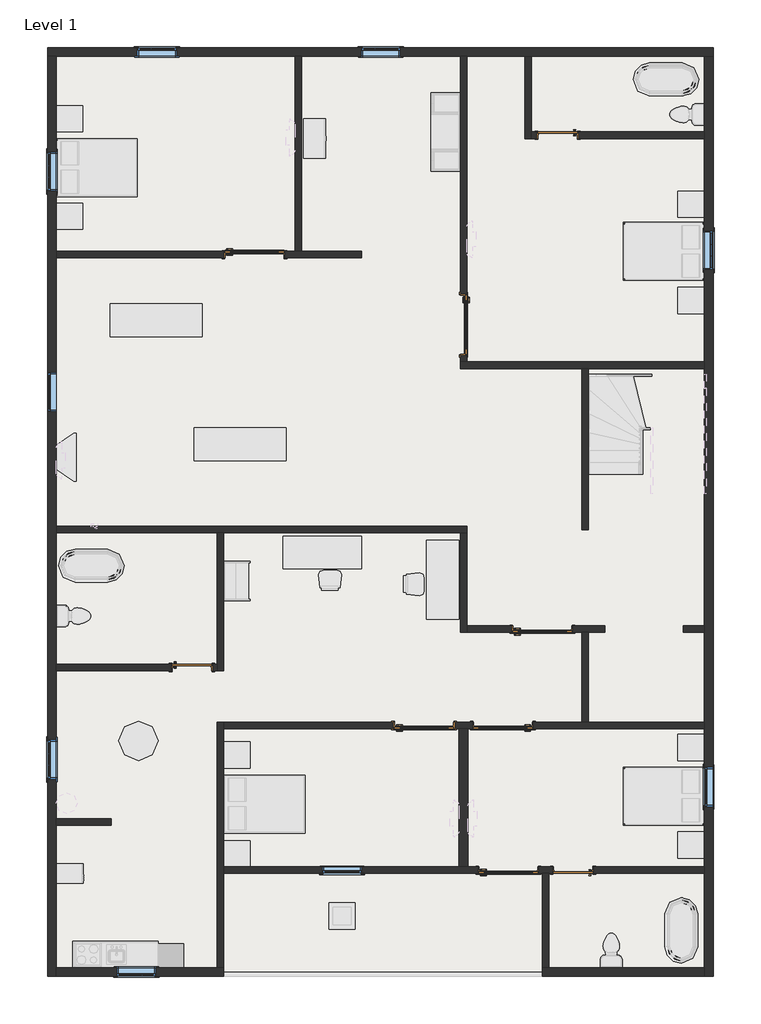
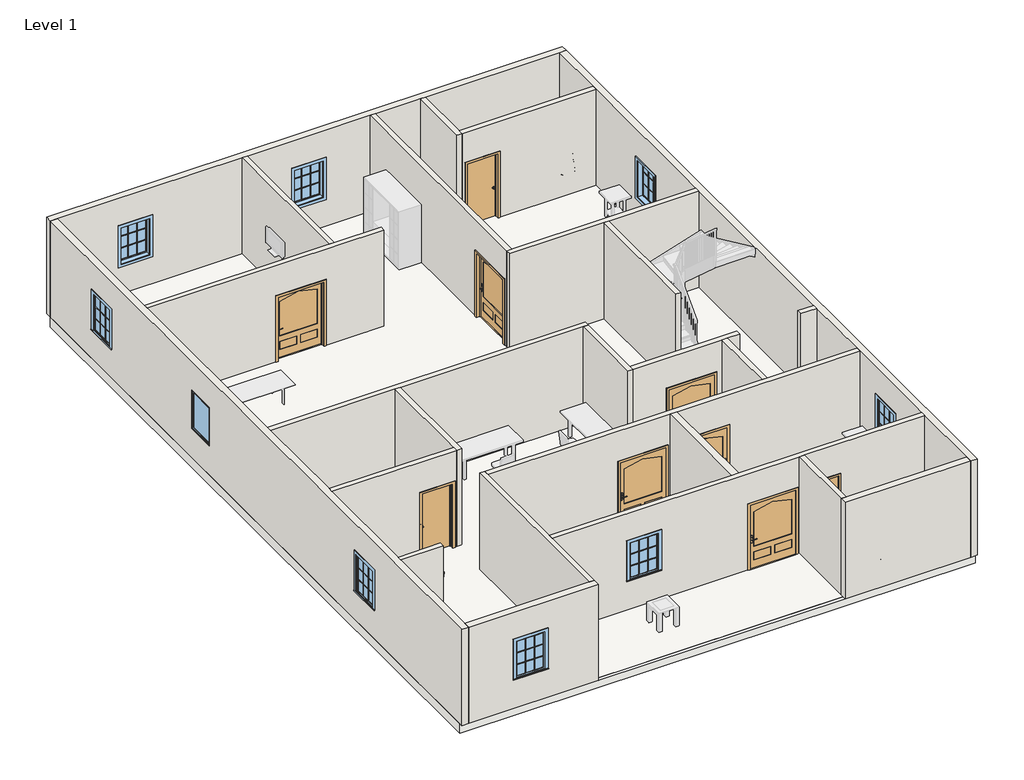
# One storey, part 1 of 2: 25 walls, 9 doors, 9 windows, 1 slab.
"""IFC4 building model written with IfcOpenShell, lengths in millimetres."""

from ifc_helpers import new_model, si_unit, frame, origin, origin_with_axes, place, context, project, spatial, polyline, outline, extrude, faceted_brep, transform, mapped, element, save
from components import door_483975e0, door_8e627b7d, door_2171c7d8, door_acdcadbb, window_29c06734, window_5c190c7e, window_e2841890

model = new_model("IFC4")

# Units and contexts
model_context = context("Model", 3, world=origin())
ifc_project = project(units=[si_unit("LENGTHUNIT", "METRE", prefix="MILLI")], contexts=[model_context])

# Site, building, storey
site = spatial("IfcSite", under=ifc_project)
building = spatial("IfcBuilding", under=site)
storey = spatial("IfcBuildingStorey", under=building, Name="Level 1", Elevation=0.0)

# Doors
placement = place(None, origin())
door_shape = door_483975e0(model_context)
element("IfcDoor", 1, ObjectType="54\" x 80\"", at=placement, inside=storey, context=model_context, shape_type="MappedRepresentation", body=[
    mapped(door_shape, transform((-4346.7860513, -470.0045948, 0.0), x_axis=(1.0, 0.0, 0.0), y_axis=(0.0, 1.0, 0.0), z_axis=(0.0, 0.0, 1.0))),
])
element("IfcDoor", 2, ObjectType="54\" x 80\"", at=placement, inside=storey, context=model_context, shape_type="MappedRepresentation", body=[
    mapped(door_shape, transform((-10112.5860513, 10458.3454052, 0.0), x_axis=(-1.0, 0.0, 0.0), y_axis=(0.0, -1.0, 0.0), z_axis=(0.0, 0.0, 1.0))),
])
element("IfcDoor", 3, ObjectType="54\" x 80\"", at=placement, inside=storey, context=model_context, shape_type="MappedRepresentation", body=[
    mapped(door_shape, transform((-5258.0110513, 8829.5704052, 0.0), x_axis=(0.0, 1.0, 0.0), y_axis=(-1.0, 0.0, 0.0), z_axis=(0.0, 0.0, 1.0))),
])
door_2_shape = door_8e627b7d(model_context)
element("IfcDoor", 4, ObjectType="54\" x 80\"", at=placement, inside=storey, context=model_context, shape_type="MappedRepresentation", body=[
    mapped(door_2_shape, transform((-4219.7860513, -3822.8045948, 0.0), x_axis=(-1.0, 0.0, 0.0), y_axis=(0.0, -1.0, 0.0), z_axis=(0.0, 0.0, 1.0))),
])
element("IfcDoor", 5, ObjectType="54\" x 80\"", at=placement, inside=storey, context=model_context, shape_type="MappedRepresentation", body=[
    mapped(door_2_shape, transform((-6175.5860513, -470.0045948, 0.0), x_axis=(-1.0, 0.0, 0.0), y_axis=(0.0, -1.0, 0.0), z_axis=(0.0, 0.0, 1.0))),
])
element("IfcDoor", 6, ObjectType="54\" x 80\"", at=placement, inside=storey, context=model_context, shape_type="MappedRepresentation", body=[
    mapped(door_2_shape, transform((-3432.3860513, 1765.1954052, 0.0), x_axis=(-1.0, 0.0, 0.0), y_axis=(0.0, -1.0, 0.0), z_axis=(0.0, 0.0, 1.0))),
])
door_3_shape = door_2171c7d8(model_context)
element("IfcDoor", 7, ObjectType="Door-Interior-Single-Flush_Panel-Wood : 36\" x 80\"", at=placement, inside=storey, context=model_context, shape_type="MappedRepresentation", body=[
    mapped(door_3_shape, transform((-2721.1860513, -3822.8045948, 0.0), x_axis=(-1.0, 0.0, 0.0), y_axis=(0.0, -1.0, 0.0), z_axis=(0.0, 0.0, 1.0))),
])
element("IfcDoor", 8, ObjectType="Door-Interior-Single-Flush_Panel-Wood : 36\" x 80\"", at=placement, inside=storey, context=model_context, shape_type="MappedRepresentation", body=[
    mapped(door_3_shape, transform((-11560.3860513, 882.5454052, 0.0), x_axis=(1.0, 0.0, 0.0), y_axis=(0.0, 1.0, 0.0), z_axis=(0.0, 0.0, 1.0))),
])
door_4_shape = door_acdcadbb(model_context)
element("IfcDoor", 9, ObjectType="Door-Interior-Single-Flush_Panel-Wood : 36\" x 80\"", at=placement, inside=storey, context=model_context, shape_type="MappedRepresentation", body=[
    mapped(door_4_shape, transform((-3076.7860513, 13226.9454052, 0.0), x_axis=(-1.0, 0.0, 0.0), y_axis=(0.0, -1.0, 0.0), z_axis=(0.0, 0.0, 1.0))),
])

# Slab
element("IfcSlab", 10, ObjectType="Generic - 12\"", at=placement, inside=storey, context=model_context, shape_type="SweptSolid", body=[
    extrude(outline(polyline([(530.0139487, 15052.5704052), (530.0139487, -6181.8295948), (-14913.1860513, -6181.8295948), (-14913.1860513, 15052.5704052), (530.0139487, 15052.5704052)])), frame((0.0, 0.0, -304.8), z_axis=(0.0, 0.0, 1.0), x_axis=(1.0, 0.0, 0.0)), (0.0, 0.0, 1.0), 304.8),
])

# Walls
element("IfcWall", 11, ObjectType="Generic - 8\"", at=placement, inside=storey, context=model_context, shape_type="Brep", body=[
    faceted_brep([(-14913.1860513, 15052.5704052, 0.0), (-14709.9860513, 15052.5704052, 0.0), (-9172.7860513, 15052.5704052, 0.0), (-9020.3860513, 15052.5704052, 0.0), (-5337.3860513, 15052.5704052, 0.0), (-5184.9860513, 15052.5704052, 0.0), (-3838.7860513, 15052.5704052, 0.0), (-3686.3860513, 15052.5704052, 0.0), (326.8139487, 15052.5704052, 0.0), (530.0139487, 15052.5704052, 0.0), (530.0139487, 15052.5704052, 3048.0), (326.8139487, 15052.5704052, 3048.0), (-3686.3860513, 15052.5704052, 3048.0), (-3838.7860513, 15052.5704052, 3048.0), (-5184.9860513, 15052.5704052, 3048.0), (-5337.3860513, 15052.5704052, 3048.0), (-9020.3860513, 15052.5704052, 3048.0), (-9172.7860513, 15052.5704052, 3048.0), (-14709.9860513, 15052.5704052, 3048.0), (-14913.1860513, 15052.5704052, 3048.0), (-11915.9860513, 15052.5704052, 2133.6), (-11915.9860513, 15052.5704052, 914.4), (-12830.3860513, 15052.5704052, 914.4), (-12830.3860513, 15052.5704052, 2133.6), (-6721.6860513, 15052.5704052, 2133.6), (-6721.6860513, 15052.5704052, 914.4), (-7636.0860513, 15052.5704052, 914.4), (-7636.0860513, 15052.5704052, 2133.6), (-14913.1860513, 15255.7704052, 0.0), (-14913.1860513, 15255.7704052, 3048.0), (530.0139487, 15255.7704052, 3048.0), (530.0139487, 15255.7704052, 0.0), (-11915.9860513, 15255.7704052, 2133.6), (-12830.3860513, 15255.7704052, 2133.6), (-12830.3860513, 15255.7704052, 914.4), (-11915.9860513, 15255.7704052, 914.4), (-6721.6860513, 15255.7704052, 2133.6), (-7636.0860513, 15255.7704052, 2133.6), (-7636.0860513, 15255.7704052, 914.4), (-6721.6860513, 15255.7704052, 914.4)], [[[0, 1, 2, 3, 4, 5, 6, 7, 8, 9, 10, 11, 12, 13, 14, 15, 16, 17, 18, 19], [20, 21, 22, 23], [24, 25, 26, 27]], [[28, 29, 30, 31], [32, 33, 34, 35], [36, 37, 38, 39]], [[9, 8, 7, 6, 5, 4, 3, 2, 1, 0, 28, 31]], [[19, 18, 17, 16, 15, 14, 13, 12, 11, 10, 30, 29]], [[10, 9, 31, 30]], [[0, 19, 29, 28]], [[21, 20, 32, 35]], [[22, 21, 35, 34]], [[23, 22, 34, 33]], [[20, 23, 33, 32]], [[25, 24, 36, 39]], [[26, 25, 39, 38]], [[27, 26, 38, 37]], [[24, 27, 37, 36]]]),
])
element("IfcWall", 12, ObjectType="Generic - 8\"", at=placement, inside=storey, context=model_context, shape_type="Brep", body=[
    faceted_brep([(326.8139487, 15052.5704052, 0.0), (326.8139487, 13299.9704052, 0.0), (326.8139487, 13147.5704052, 0.0), (326.8139487, 7965.9704052, 0.0), (326.8139487, 7813.5704052, 0.0), (326.8139487, 1844.5704052, 0.0), (326.8139487, 1692.1704052, 0.0), (326.8139487, -390.6295948, 0.0), (326.8139487, -543.0295948, 0.0), (326.8139487, -3743.4295948, 0.0), (326.8139487, -3895.8295948, 0.0), (326.8139487, -6080.2295948, 0.0), (326.8139487, -6283.4295948, 0.0), (326.8139487, -6283.4295948, 3048.0), (326.8139487, -6080.2295948, 3048.0), (326.8139487, -3895.8295948, 3048.0), (326.8139487, -3743.4295948, 3048.0), (326.8139487, -543.0295948, 3048.0), (326.8139487, -390.6295948, 3048.0), (326.8139487, 1692.1704052, 3048.0), (326.8139487, 1844.5704052, 3048.0), (326.8139487, 7813.5704052, 3048.0), (326.8139487, 7965.9704052, 3048.0), (326.8139487, 13147.5704052, 3048.0), (326.8139487, 13299.9704052, 3048.0), (326.8139487, 15052.5704052, 3048.0), (326.8139487, -1432.0295948, 2133.6), (326.8139487, -2346.4295948, 2133.6), (326.8139487, -2346.4295948, 914.4), (326.8139487, -1432.0295948, 914.4), (326.8139487, 10099.5704052, 2133.6), (326.8139487, 10099.5704052, 914.4), (326.8139487, 11013.9704052, 914.4), (326.8139487, 11013.9704052, 2133.6), (530.0139487, 15052.5704052, 0.0), (530.0139487, 15052.5704052, 3048.0), (530.0139487, -6283.4295948, 3048.0), (530.0139487, -6283.4295948, 0.0), (530.0139487, -1432.0295948, 2133.6), (530.0139487, -1432.0295948, 914.4), (530.0139487, -2346.4295948, 914.4), (530.0139487, -2346.4295948, 2133.6), (530.0139487, 10099.5704052, 2133.6), (530.0139487, 11013.9704052, 2133.6), (530.0139487, 11013.9704052, 914.4), (530.0139487, 10099.5704052, 914.4)], [[[0, 1, 2, 3, 4, 5, 6, 7, 8, 9, 10, 11, 12, 13, 14, 15, 16, 17, 18, 19, 20, 21, 22, 23, 24, 25], [26, 27, 28, 29], [30, 31, 32, 33]], [[34, 35, 36, 37], [38, 39, 40, 41], [42, 43, 44, 45]], [[12, 11, 10, 9, 8, 7, 6, 5, 4, 3, 2, 1, 0, 34, 37]], [[25, 24, 23, 22, 21, 20, 19, 18, 17, 16, 15, 14, 13, 36, 35]], [[0, 25, 35, 34]], [[13, 12, 37, 36]], [[39, 38, 26, 29]], [[40, 39, 29, 28]], [[41, 40, 28, 27]], [[38, 41, 27, 26]], [[31, 30, 42, 45]], [[32, 31, 45, 44]], [[33, 32, 44, 43]], [[30, 33, 43, 42]]]),
])
element("IfcWall", 13, ObjectType="Generic - 8\"", at=placement, inside=storey, context=model_context, shape_type="Brep", body=[
    faceted_brep([(-14913.1860513, 15052.5704052, 0.0), (-14913.1860513, -6283.4295948, 0.0), (-14913.1860513, -6283.4295948, 3048.0), (-14913.1860513, 15052.5704052, 3048.0), (-14913.1860513, 12842.7704052, 2133.6), (-14913.1860513, 11928.3704052, 2133.6), (-14913.1860513, 11928.3704052, 914.4), (-14913.1860513, 12842.7704052, 914.4), (-14913.1860513, -797.0295948, 2133.6), (-14913.1860513, -1711.4295948, 2133.6), (-14913.1860513, -1711.4295948, 914.4), (-14913.1860513, -797.0295948, 914.4), (-14913.1860513, 7724.6704052, 2133.6), (-14913.1860513, 6810.2704052, 2133.6), (-14913.1860513, 6810.2704052, 914.4), (-14913.1860513, 7724.6704052, 914.4), (-14709.9860513, 15052.5704052, 0.0), (-14709.9860513, 15052.5704052, 3048.0), (-14709.9860513, 10531.3704052, 3048.0), (-14709.9860513, 10378.9704052, 3048.0), (-14709.9860513, 4155.9704052, 3048.0), (-14709.9860513, 4003.5704052, 3048.0), (-14709.9860513, 955.5704052, 3048.0), (-14709.9860513, 803.1704052, 3048.0), (-14709.9860513, -2625.8295948, 3048.0), (-14709.9860513, -2778.2295948, 3048.0), (-14709.9860513, -6080.2295948, 3048.0), (-14709.9860513, -6283.4295948, 3048.0), (-14709.9860513, -6283.4295948, 0.0), (-14709.9860513, -6080.2295948, 0.0), (-14709.9860513, -2778.2295948, 0.0), (-14709.9860513, -2625.8295948, 0.0), (-14709.9860513, 803.1704052, 0.0), (-14709.9860513, 955.5704052, 0.0), (-14709.9860513, 4003.5704052, 0.0), (-14709.9860513, 4155.9704052, 0.0), (-14709.9860513, 10378.9704052, 0.0), (-14709.9860513, 10531.3704052, 0.0), (-14709.9860513, 12842.7704052, 2133.6), (-14709.9860513, 12842.7704052, 914.4), (-14709.9860513, 11928.3704052, 914.4), (-14709.9860513, 11928.3704052, 2133.6), (-14709.9860513, -797.0295948, 2133.6), (-14709.9860513, -797.0295948, 914.4), (-14709.9860513, -1711.4295948, 914.4), (-14709.9860513, -1711.4295948, 2133.6), (-14709.9860513, 7724.6704052, 2133.6), (-14709.9860513, 7724.6704052, 914.4), (-14709.9860513, 6810.2704052, 914.4), (-14709.9860513, 6810.2704052, 2133.6)], [[[0, 1, 2, 3], [4, 5, 6, 7], [8, 9, 10, 11], [12, 13, 14, 15]], [[16, 17, 18, 19, 20, 21, 22, 23, 24, 25, 26, 27, 28, 29, 30, 31, 32, 33, 34, 35, 36, 37], [38, 39, 40, 41], [42, 43, 44, 45], [46, 47, 48, 49]], [[1, 0, 16, 37, 36, 35, 34, 33, 32, 31, 30, 29, 28]], [[3, 2, 27, 26, 25, 24, 23, 22, 21, 20, 19, 18, 17]], [[0, 3, 17, 16]], [[2, 1, 28, 27]], [[39, 38, 4, 7]], [[40, 39, 7, 6]], [[41, 40, 6, 5]], [[38, 41, 5, 4]], [[43, 42, 8, 11]], [[44, 43, 11, 10]], [[45, 44, 10, 9]], [[42, 45, 9, 8]], [[47, 46, 12, 15]], [[48, 47, 15, 14]], [[49, 48, 14, 13]], [[46, 49, 13, 12]]]),
])
element("IfcWall", 14, ObjectType="Generic - 8\"", at=placement, inside=storey, context=model_context, shape_type="Brep", body=[
    faceted_brep([(-14709.9860513, -6283.4295948, 0.0), (-10823.7860513, -6283.4295948, 0.0), (-10823.7860513, -6283.4295948, 3048.0), (-14709.9860513, -6283.4295948, 3048.0), (-13312.9860513, -6283.4295948, 2133.6), (-12398.5860513, -6283.4295948, 2133.6), (-12398.5860513, -6283.4295948, 914.4), (-13312.9860513, -6283.4295948, 914.4), (-14709.9860513, -6080.2295948, 0.0), (-14709.9860513, -6080.2295948, 3048.0), (-10976.1860513, -6080.2295948, 3048.0), (-10823.7860513, -6080.2295948, 3048.0), (-10823.7860513, -6080.2295948, 0.0), (-10976.1860513, -6080.2295948, 0.0), (-13312.9860513, -6080.2295948, 2133.6), (-13312.9860513, -6080.2295948, 914.4), (-12398.5860513, -6080.2295948, 914.4), (-12398.5860513, -6080.2295948, 2133.6)], [[[0, 1, 2, 3], [4, 5, 6, 7]], [[8, 9, 10, 11, 12, 13], [14, 15, 16, 17]], [[1, 0, 8, 13, 12]], [[3, 2, 11, 10, 9]], [[0, 3, 9, 8]], [[2, 1, 12, 11]], [[15, 14, 4, 7]], [[16, 15, 7, 6]], [[17, 16, 6, 5]], [[14, 17, 5, 4]]]),
])
element("IfcWall", 15, ObjectType="Generic - 8\"", at=placement, inside=storey, context=model_context, shape_type="SweptSolid", body=[
    extrude(outline(polyline([(-5362.7860513, -3743.4295948), (-5362.7860513, -543.0295948), (-5159.5860513, -543.0295948), (-5159.5860513, -3743.4295948), (-5362.7860513, -3743.4295948)])), origin_with_axes(), (0.0, 0.0, 1.0), 3048.0),
])
element("IfcWall", 16, ObjectType="Generic - 8\"", at=placement, inside=storey, context=model_context, shape_type="Brep", body=[
    faceted_brep([(-3432.3860513, -6283.4295948, 0.0), (326.8139487, -6283.4295948, 0.0), (326.8139487, -6283.4295948, 3048.0), (-3432.3860513, -6283.4295948, 3048.0), (-3432.3860513, -6080.2295948, 0.0), (-3432.3860513, -6080.2295948, 3048.0), (-3279.9860513, -6080.2295948, 3048.0), (326.8139487, -6080.2295948, 3048.0), (326.8139487, -6080.2295948, 0.0), (-3279.9860513, -6080.2295948, 0.0)], [[[0, 1, 2, 3]], [[4, 5, 6, 7, 8, 9]], [[1, 0, 4, 9, 8]], [[3, 2, 7, 6, 5]], [[2, 1, 8, 7]], [[0, 3, 5, 4]]]),
])
element("IfcWall", 17, ObjectType="INNER WALL", at=placement, inside=storey, context=model_context, shape_type="SweptSolid", body=[
    extrude(outline(polyline([(-9172.7860513, 10531.3704052), (-9172.7860513, 15052.5704052), (-9020.3860513, 15052.5704052), (-9020.3860513, 10531.3704052), (-9172.7860513, 10531.3704052)])), origin_with_axes(), (0.0, 0.0, 1.0), 3048.0),
])
element("IfcWall", 18, ObjectType="INNER WALL", at=placement, inside=storey, context=model_context, shape_type="Brep", body=[
    faceted_brep([(-14709.9860513, 10531.3704052, 3048.0), (-9172.7860513, 10531.3704052, 3048.0), (-9020.3860513, 10531.3704052, 3048.0), (-7623.3860513, 10531.3704052, 3048.0), (-7623.3860513, 10531.3704052, 0.0), (-9020.3860513, 10531.3704052, 0.0), (-9172.7860513, 10531.3704052, 0.0), (-9401.3860513, 10531.3704052, 0.0), (-9401.3860513, 10531.3704052, 2057.4), (-10823.7860513, 10531.3704052, 2057.4), (-10823.7860513, 10531.3704052, 0.0), (-14709.9860513, 10531.3704052, 0.0), (-7623.3860513, 10378.9704052, 3048.0), (-14709.9860513, 10378.9704052, 3048.0), (-14709.9860513, 10378.9704052, 0.0), (-10823.7860513, 10378.9704052, 0.0), (-10823.7860513, 10378.9704052, 2057.4), (-9401.3860513, 10378.9704052, 2057.4), (-9401.3860513, 10378.9704052, 0.0), (-7623.3860513, 10378.9704052, 0.0)], [[[0, 1, 2, 3, 4, 5, 6, 7, 8, 9, 10, 11]], [[12, 13, 14, 15, 16, 17, 18, 19]], [[4, 19, 18, 7, 6, 5]], [[14, 11, 10, 15]], [[3, 2, 1, 0, 13, 12]], [[4, 3, 12, 19]], [[0, 11, 14, 13]], [[9, 16, 15, 10]], [[16, 9, 8, 17]], [[17, 8, 7, 18]]]),
])
element("IfcWall", 19, ObjectType="INNER WALL", at=placement, inside=storey, context=model_context, shape_type="SweptSolid", body=[
    extrude(outline(polyline([(7965.9704052, 3048.0), (15052.5704052, 3048.0), (15052.5704052, 0.0), (9540.7704052, 0.0), (9540.7704052, 2057.4), (8118.3704052, 2057.4), (8118.3704052, 0.0), (7965.9704052, 0.0), (7965.9704052, 3048.0)])), frame((-5337.3860513, 0.0, 0.0), z_axis=(1.0, 0.0, 0.0), x_axis=(0.0, 1.0, 0.0)), (0.0, 0.0, 1.0), 152.4),
])
element("IfcWall", 20, ObjectType="INNER WALL", at=placement, inside=storey, context=model_context, shape_type="Brep", body=[
    faceted_brep([(-5337.3860513, 7813.5704052, 0.0), (-2517.9860513, 7813.5704052, 0.0), (-2365.5860513, 7813.5704052, 0.0), (326.8139487, 7813.5704052, 0.0), (326.8139487, 7813.5704052, 3048.0), (-2365.5860513, 7813.5704052, 3048.0), (-2517.9860513, 7813.5704052, 3048.0), (-5337.3860513, 7813.5704052, 3048.0), (-5337.3860513, 7965.9704052, 0.0), (-5337.3860513, 7965.9704052, 3048.0), (-5184.9860513, 7965.9704052, 3048.0), (326.8139487, 7965.9704052, 3048.0), (326.8139487, 7965.9704052, 0.0), (-5184.9860513, 7965.9704052, 0.0)], [[[0, 1, 2, 3, 4, 5, 6, 7]], [[8, 9, 10, 11, 12, 13]], [[3, 2, 1, 0, 8, 13, 12]], [[7, 6, 5, 4, 11, 10, 9]], [[4, 3, 12, 11]], [[0, 7, 9, 8]]]),
])
element("IfcWall", 21, ObjectType="INNER WALL", at=placement, inside=storey, context=model_context, shape_type="SweptSolid", body=[
    extrude(outline(polyline([(-2517.9860513, 4079.7704052), (-2517.9860513, 7813.5704052), (-2365.5860513, 7813.5704052), (-2365.5860513, 4079.7704052), (-2517.9860513, 4079.7704052)])), origin_with_axes(), (0.0, 0.0, 1.0), 3048.0),
])
element("IfcWall", 22, ObjectType="INNER WALL", at=placement, inside=storey, context=model_context, shape_type="Brep", body=[
    faceted_brep([(-14709.9860513, 4003.5704052, 0.0), (-10976.1860513, 4003.5704052, 0.0), (-10823.7860513, 4003.5704052, 0.0), (-5337.3860513, 4003.5704052, 0.0), (-5184.9860513, 4003.5704052, 0.0), (-5184.9860513, 4003.5704052, 3048.0), (-5337.3860513, 4003.5704052, 3048.0), (-10823.7860513, 4003.5704052, 3048.0), (-10976.1860513, 4003.5704052, 3048.0), (-14709.9860513, 4003.5704052, 3048.0), (-14709.9860513, 4155.9704052, 0.0), (-14709.9860513, 4155.9704052, 3048.0), (-5184.9860513, 4155.9704052, 3048.0), (-5184.9860513, 4155.9704052, 0.0)], [[[0, 1, 2, 3, 4, 5, 6, 7, 8, 9]], [[10, 11, 12, 13]], [[4, 3, 2, 1, 0, 10, 13]], [[9, 8, 7, 6, 5, 12, 11]], [[0, 9, 11, 10]], [[5, 4, 13, 12]]]),
])
element("IfcWall", 23, ObjectType="INNER WALL", at=placement, inside=storey, context=model_context, shape_type="Brep", body=[
    faceted_brep([(-5337.3860513, 4003.5704052, 0.0), (-5337.3860513, 1692.1704052, 0.0), (-5337.3860513, 1692.1704052, 3048.0), (-5337.3860513, 4003.5704052, 3048.0), (-5184.9860513, 4003.5704052, 0.0), (-5184.9860513, 4003.5704052, 3048.0), (-5184.9860513, 1844.5704052, 3048.0), (-5184.9860513, 1692.1704052, 3048.0), (-5184.9860513, 1692.1704052, 0.0), (-5184.9860513, 1844.5704052, 0.0)], [[[0, 1, 2, 3]], [[4, 5, 6, 7, 8, 9]], [[1, 0, 4, 9, 8]], [[3, 2, 7, 6, 5]], [[0, 3, 5, 4]], [[2, 1, 8, 7]]]),
])
element("IfcWall", 24, ObjectType="INNER WALL", at=placement, inside=storey, context=model_context, shape_type="Brep", body=[
    faceted_brep([(-1984.5860513, 1692.1704052, 0.0), (-1984.5860513, 1692.1704052, 3048.0), (-2365.5860513, 1692.1704052, 3048.0), (-2517.9860513, 1692.1704052, 3048.0), (-5184.9860513, 1692.1704052, 3048.0), (-5184.9860513, 1692.1704052, 0.0), (-4143.5860513, 1692.1704052, 0.0), (-4143.5860513, 1692.1704052, 2057.4), (-2721.1860513, 1692.1704052, 2057.4), (-2721.1860513, 1692.1704052, 0.0), (-2517.9860513, 1692.1704052, 0.0), (-2365.5860513, 1692.1704052, 0.0), (-1984.5860513, 1844.5704052, 3048.0), (-1984.5860513, 1844.5704052, 0.0), (-2721.1860513, 1844.5704052, 0.0), (-2721.1860513, 1844.5704052, 2057.4), (-4143.5860513, 1844.5704052, 2057.4), (-4143.5860513, 1844.5704052, 0.0), (-5184.9860513, 1844.5704052, 0.0), (-5184.9860513, 1844.5704052, 3048.0)], [[[0, 1, 2, 3, 4, 5, 6, 7, 8, 9, 10, 11]], [[12, 13, 14, 15, 16, 17, 18, 19]], [[13, 0, 11, 10, 9, 14]], [[5, 18, 17, 6]], [[1, 0, 13, 12]], [[4, 3, 2, 1, 12, 19]], [[5, 4, 19, 18]], [[16, 7, 6, 17]], [[7, 16, 15, 8]], [[8, 15, 14, 9]]]),
])
element("IfcWall", 25, ObjectType="INNER WALL", at=placement, inside=storey, context=model_context, shape_type="SweptSolid", body=[
    extrude(outline(polyline([(-2517.9860513, -390.6295948), (-2517.9860513, 1692.1704052), (-2365.5860513, 1692.1704052), (-2365.5860513, -390.6295948), (-2517.9860513, -390.6295948)])), origin_with_axes(), (0.0, 0.0, 1.0), 3048.0),
])
element("IfcWall", 26, ObjectType="INNER WALL", at=placement, inside=storey, context=model_context, shape_type="SweptSolid", body=[
    extrude(outline(polyline([(-3279.9860513, -3895.8295948), (-3279.9860513, -6080.2295948), (-3432.3860513, -6080.2295948), (-3432.3860513, -3895.8295948), (-3279.9860513, -3895.8295948)])), origin_with_axes(), (0.0, 0.0, 1.0), 3048.0),
])
element("IfcWall", 27, ObjectType="INNER WALL", at=placement, inside=storey, context=model_context, shape_type="Brep", body=[
    faceted_brep([(-10823.7860513, -6080.2295948, 0.0), (-10823.7860513, -3895.8295948, 0.0), (-10823.7860513, -3743.4295948, 0.0), (-10823.7860513, -543.0295948, 0.0), (-10823.7860513, -390.6295948, 0.0), (-10823.7860513, -390.6295948, 3048.0), (-10823.7860513, -543.0295948, 3048.0), (-10823.7860513, -3743.4295948, 3048.0), (-10823.7860513, -3895.8295948, 3048.0), (-10823.7860513, -6080.2295948, 3048.0), (-10976.1860513, -6080.2295948, 0.0), (-10976.1860513, -6080.2295948, 3048.0), (-10976.1860513, -390.6295948, 3048.0), (-10976.1860513, -390.6295948, 0.0)], [[[0, 1, 2, 3, 4, 5, 6, 7, 8, 9]], [[10, 11, 12, 13]], [[4, 3, 2, 1, 0, 10, 13]], [[9, 8, 7, 6, 5, 12, 11]], [[5, 4, 13, 12]], [[0, 9, 11, 10]]]),
])
element("IfcWall", 28, ObjectType="INNER WALL", at=placement, inside=storey, context=model_context, shape_type="Brep", body=[
    faceted_brep([(326.8139487, -543.0295948, 3048.0), (-5159.5860513, -543.0295948, 3048.0), (-5362.7860513, -543.0295948, 3048.0), (-10823.7860513, -543.0295948, 3048.0), (-10823.7860513, -543.0295948, 0.0), (-6886.7860513, -543.0295948, 0.0), (-6886.7860513, -543.0295948, 2057.4), (-5464.3860513, -543.0295948, 2057.4), (-5464.3860513, -543.0295948, 0.0), (-5362.7860513, -543.0295948, 0.0), (-5159.5860513, -543.0295948, 0.0), (-5057.9860513, -543.0295948, 0.0), (-5057.9860513, -543.0295948, 2057.4), (-3635.5860513, -543.0295948, 2057.4), (-3635.5860513, -543.0295948, 0.0), (326.8139487, -543.0295948, 0.0), (-10823.7860513, -390.6295948, 3048.0), (-2517.9860513, -390.6295948, 3048.0), (-2365.5860513, -390.6295948, 3048.0), (326.8139487, -390.6295948, 3048.0), (326.8139487, -390.6295948, 0.0), (-2365.5860513, -390.6295948, 0.0), (-2517.9860513, -390.6295948, 0.0), (-3635.5860513, -390.6295948, 0.0), (-3635.5860513, -390.6295948, 2057.4), (-5057.9860513, -390.6295948, 2057.4), (-5057.9860513, -390.6295948, 0.0), (-5464.3860513, -390.6295948, 0.0), (-5464.3860513, -390.6295948, 2057.4), (-6886.7860513, -390.6295948, 2057.4), (-6886.7860513, -390.6295948, 0.0), (-10823.7860513, -390.6295948, 0.0)], [[[0, 1, 2, 3, 4, 5, 6, 7, 8, 9, 10, 11, 12, 13, 14, 15]], [[16, 17, 18, 19, 20, 21, 22, 23, 24, 25, 26, 27, 28, 29, 30, 31]], [[4, 31, 30, 5]], [[20, 15, 14, 23, 22, 21]], [[26, 11, 10, 9, 8, 27]], [[3, 2, 1, 0, 19, 18, 17, 16]], [[4, 3, 16, 31]], [[0, 15, 20, 19]], [[13, 24, 23, 14]], [[24, 13, 12, 25]], [[25, 12, 11, 26]], [[29, 6, 5, 30]], [[6, 29, 28, 7]], [[7, 28, 27, 8]]]),
])
element("IfcWall", 29, ObjectType="INNER WALL", at=placement, inside=storey, context=model_context, shape_type="Brep", body=[
    faceted_brep([(-10823.7860513, -3743.4295948, 3048.0), (-5362.7860513, -3743.4295948, 3048.0), (-5159.5860513, -3743.4295948, 3048.0), (326.8139487, -3743.4295948, 3048.0), (326.8139487, -3743.4295948, 0.0), (-2238.5860513, -3743.4295948, 0.0), (-2238.5860513, -3743.4295948, 2057.4), (-3203.7860513, -3743.4295948, 2057.4), (-3203.7860513, -3743.4295948, 0.0), (-3508.5860513, -3743.4295948, 0.0), (-3508.5860513, -3743.4295948, 2057.4), (-4930.9860513, -3743.4295948, 2057.4), (-4930.9860513, -3743.4295948, 0.0), (-5159.5860513, -3743.4295948, 0.0), (-5362.7860513, -3743.4295948, 0.0), (-10823.7860513, -3743.4295948, 0.0), (-8537.7860513, -3743.4295948, 2133.6), (-8537.7860513, -3743.4295948, 914.4), (-7623.3860513, -3743.4295948, 914.4), (-7623.3860513, -3743.4295948, 2133.6), (326.8139487, -3895.8295948, 3048.0), (-3279.9860513, -3895.8295948, 3048.0), (-3432.3860513, -3895.8295948, 3048.0), (-10823.7860513, -3895.8295948, 3048.0), (-10823.7860513, -3895.8295948, 0.0), (-4930.9860513, -3895.8295948, 0.0), (-4930.9860513, -3895.8295948, 2057.4), (-3508.5860513, -3895.8295948, 2057.4), (-3508.5860513, -3895.8295948, 0.0), (-3432.3860513, -3895.8295948, 0.0), (-3279.9860513, -3895.8295948, 0.0), (-3203.7860513, -3895.8295948, 0.0), (-3203.7860513, -3895.8295948, 2057.4), (-2238.5860513, -3895.8295948, 2057.4), (-2238.5860513, -3895.8295948, 0.0), (326.8139487, -3895.8295948, 0.0), (-8537.7860513, -3895.8295948, 2133.6), (-7623.3860513, -3895.8295948, 2133.6), (-7623.3860513, -3895.8295948, 914.4), (-8537.7860513, -3895.8295948, 914.4)], [[[0, 1, 2, 3, 4, 5, 6, 7, 8, 9, 10, 11, 12, 13, 14, 15], [16, 17, 18, 19]], [[20, 21, 22, 23, 24, 25, 26, 27, 28, 29, 30, 31, 32, 33, 34, 35], [36, 37, 38, 39]], [[24, 15, 14, 13, 12, 25]], [[4, 35, 34, 5]], [[28, 9, 8, 31, 30, 29]], [[3, 2, 1, 0, 23, 22, 21, 20]], [[0, 15, 24, 23]], [[4, 3, 20, 35]], [[11, 26, 25, 12]], [[26, 11, 10, 27]], [[27, 10, 9, 28]], [[7, 32, 31, 8]], [[32, 7, 6, 33]], [[33, 6, 5, 34]], [[17, 16, 36, 39]], [[18, 17, 39, 38]], [[19, 18, 38, 37]], [[16, 19, 37, 36]]]),
])
element("IfcWall", 30, ObjectType="INNER WALL", at=placement, inside=storey, context=model_context, shape_type="Brep", body=[
    faceted_brep([(-10976.1860513, 4003.5704052, 0.0), (-10976.1860513, 955.5704052, 0.0), (-10976.1860513, 803.1704052, 0.0), (-10976.1860513, 803.1704052, 3048.0), (-10976.1860513, 955.5704052, 3048.0), (-10976.1860513, 4003.5704052, 3048.0), (-10823.7860513, 4003.5704052, 0.0), (-10823.7860513, 4003.5704052, 3048.0), (-10823.7860513, 803.1704052, 3048.0), (-10823.7860513, 803.1704052, 0.0)], [[[0, 1, 2, 3, 4, 5]], [[6, 7, 8, 9]], [[2, 1, 0, 6, 9]], [[5, 4, 3, 8, 7]], [[0, 5, 7, 6]], [[3, 2, 9, 8]]]),
])
element("IfcWall", 31, ObjectType="INNER WALL", at=placement, inside=storey, context=model_context, shape_type="SweptSolid", body=[
    extrude(outline(polyline([(3048.0, -10976.1860513), (3048.0, -14709.9860513), (0.0, -14709.9860513), (0.0, -12042.9860513), (2057.4, -12042.9860513), (2057.4, -11077.7860513), (0.0, -11077.7860513), (0.0, -10976.1860513), (3048.0, -10976.1860513)])), frame((0.0, 803.1704052, 0.0), z_axis=(0.0, 1.0, 0.0), x_axis=(0.0, 0.0, 1.0)), (0.0, 0.0, 1.0), 152.4),
])
element("IfcWall", 32, ObjectType="INNER WALL", at=placement, inside=storey, context=model_context, shape_type="SweptSolid", body=[
    extrude(outline(polyline([(326.8139487, 1692.1704052), (-155.7860513, 1692.1704052), (-155.7860513, 1844.5704052), (326.8139487, 1844.5704052), (326.8139487, 1692.1704052)])), origin_with_axes(), (0.0, 0.0, 1.0), 3048.0),
])
element("IfcWall", 33, ObjectType="INNER WALL", at=placement, inside=storey, context=model_context, shape_type="Brep", body=[
    faceted_brep([(-3838.7860513, 15052.5704052, 0.0), (-3838.7860513, 13147.5704052, 0.0), (-3838.7860513, 13147.5704052, 3048.0), (-3838.7860513, 15052.5704052, 3048.0), (-3686.3860513, 15052.5704052, 0.0), (-3686.3860513, 15052.5704052, 3048.0), (-3686.3860513, 13299.9704052, 3048.0), (-3686.3860513, 13147.5704052, 3048.0), (-3686.3860513, 13147.5704052, 0.0), (-3686.3860513, 13299.9704052, 0.0)], [[[0, 1, 2, 3]], [[4, 5, 6, 7, 8, 9]], [[1, 0, 4, 9, 8]], [[3, 2, 7, 6, 5]], [[0, 3, 5, 4]], [[2, 1, 8, 7]]]),
])
element("IfcWall", 34, ObjectType="INNER WALL", at=placement, inside=storey, context=model_context, shape_type="SweptSolid", body=[
    extrude(outline(polyline([(3048.0, 326.8139487), (3048.0, -3686.3860513), (0.0, -3686.3860513), (0.0, -3559.3860513), (2057.4, -3559.3860513), (2057.4, -2594.1860513), (0.0, -2594.1860513), (0.0, 326.8139487), (3048.0, 326.8139487)])), frame((0.0, 13147.5704052, 0.0), z_axis=(0.0, 1.0, 0.0), x_axis=(0.0, 0.0, 1.0)), (0.0, 0.0, 1.0), 152.4),
])
element("IfcWall", 35, ObjectType="INNER WALL", at=placement, inside=storey, context=model_context, shape_type="SweptSolid", body=[
    extrude(outline(polyline([(-14709.9860513, -2625.8295948), (-13439.9860513, -2625.8295948), (-13439.9860513, -2778.2295948), (-14709.9860513, -2778.2295948), (-14709.9860513, -2625.8295948)])), origin_with_axes(), (0.0, 0.0, 1.0), 3048.0),
])

# Windows
window_shape = window_29c06734(model_context)
element("IfcWindow", 36, ObjectType="Casement 3x3 with Trim : 36\" x 48\"", at=placement, inside=storey, context=model_context, shape_type="MappedRepresentation", body=[
    mapped(window_shape, transform((-12855.7860513, -6181.8295948, 0.0), x_axis=(-1.0, 0.0, 0.0), y_axis=(0.0, -1.0, 0.0), z_axis=(0.0, 0.0, 1.0))),
])
element("IfcWindow", 37, ObjectType="Casement 3x3 with Trim : 36\" x 48\"", at=placement, inside=storey, context=model_context, shape_type="MappedRepresentation", body=[
    mapped(window_shape, transform((428.4139487, -1889.2295948, 0.0), x_axis=(0.0, 1.0, 0.0), y_axis=(-1.0, 0.0, 0.0), z_axis=(0.0, 0.0, 1.0))),
])
element("IfcWindow", 38, ObjectType="Casement 3x3 with Trim : 36\" x 48\"", at=placement, inside=storey, context=model_context, shape_type="MappedRepresentation", body=[
    mapped(window_shape, transform((428.4139487, 10556.7704052, 0.0), x_axis=(0.0, -1.0, 0.0), y_axis=(1.0, 0.0, 0.0), z_axis=(0.0, 0.0, 1.0))),
])
element("IfcWindow", 39, ObjectType="Casement 3x3 with Trim : 36\" x 48\"", at=placement, inside=storey, context=model_context, shape_type="MappedRepresentation", body=[
    mapped(window_shape, transform((-12373.1860513, 15154.1704052, 0.0), x_axis=(1.0, 0.0, 0.0), y_axis=(0.0, 1.0, 0.0), z_axis=(0.0, 0.0, 1.0))),
])
element("IfcWindow", 40, ObjectType="Casement 3x3 with Trim : 36\" x 48\"", at=placement, inside=storey, context=model_context, shape_type="MappedRepresentation", body=[
    mapped(window_shape, transform((-14811.5860513, 12385.5704052, 0.0), x_axis=(0.0, 1.0, 0.0), y_axis=(-1.0, 0.0, 0.0), z_axis=(0.0, 0.0, 1.0))),
])
element("IfcWindow", 41, ObjectType="Casement 3x3 with Trim : 36\" x 48\"", at=placement, inside=storey, context=model_context, shape_type="MappedRepresentation", body=[
    mapped(window_shape, transform((-14811.5860513, -1254.2295948, 0.0), x_axis=(0.0, 1.0, 0.0), y_axis=(-1.0, 0.0, 0.0), z_axis=(0.0, 0.0, 1.0))),
])
element("IfcWindow", 42, ObjectType="Casement 3x3 with Trim : 36\" x 48\"", at=placement, inside=storey, context=model_context, shape_type="MappedRepresentation", body=[
    mapped(window_shape, transform((-7178.8860513, 15154.1704052, 0.0), x_axis=(1.0, 0.0, 0.0), y_axis=(0.0, 1.0, 0.0), z_axis=(0.0, 0.0, 1.0))),
])
window_2_shape = window_5c190c7e(model_context)
element("IfcWindow", 43, ObjectType="Casement 3x3 with Trim : 36\" x 48\"", at=placement, inside=storey, context=model_context, shape_type="MappedRepresentation", body=[
    mapped(window_2_shape, transform((-8080.5860513, -3819.6295948, 0.0), x_axis=(-1.0, 0.0, 0.0), y_axis=(0.0, -1.0, 0.0), z_axis=(0.0, 0.0, 1.0))),
])
window_3_shape = window_e2841890(model_context)
element("IfcWindow", 44, ObjectType="Fixed : 36\" x 48\"", at=placement, inside=storey, context=model_context, shape_type="MappedRepresentation", body=[
    mapped(window_3_shape, transform((-14811.5860513, 7305.5704052, 0.0), x_axis=(0.0, 1.0, 0.0), y_axis=(-1.0, 0.0, 0.0), z_axis=(0.0, 0.0, 1.0))),
])

save(model, "model.ifc")

# Revit data of these elements
# Type "54\" x 80\""
#   Type Mark = "8"
#   Assembly Code = "B2030100"
#   Analytic Construction = "French door, wood frame with single glass"
#   Threshold Offset [instance default] = 0' - 0 1/2"
#   Thickness = 0' - 1 3/8"
#   Thermal Resistance (R) = 1.0696 (h·ft²·°F)/BTU
#   Swing Angle [instance default] = 90.00°
#   Stiles = 0' - 4 3/4"
#   Rough Width = 4' - 8"
#   Rough Height = 6' - 9"
#   Radius = 4' - 4.00625"
#   Lock Rail = 0' - 7 1/8"
#   Height = 6' - 8"
#   Width = 4' - 6"
#   Heat Transfer Coefficient (U) = 0.9350 BTU/(h·ft²·°F)
#   Door Offset [instance default] = 0' - 0"
#   Bottom Rail = 0' - 9 1/2"
#   Threshold [instance default] = yes
#   Function = 1
#   Exterior Trim [instance default] = yes
#   Trim Material = Cherry
#   Threshold Material = Cherry
#   Panel Material = Cherry
#   Glazing = Glass
#   Frame Material = Cherry
#   Door Handle Material = Aluminum
#   Visual Light Transmittance = 0
#   Solar Heat Gain Coefficient = 0
#   Wall Closure = (empty or 0)
#   Construction Type = (empty or 0)
# Type "Door-Interior-Single-Flush_Panel-Wood : 36\" x 80\""
#   Type Mark = "9"
#   Assembly Code = "C1020300"
#   Analytic Construction = "Wooden"
#   Thickness = 0' - 1 3/8"
#   Thermal Resistance (R) = 2.5876 (h·ft²·°F)/BTU
#   Swing Angle [instance default] = 90.00°
#   Rough Width = 3' - 2"
#   Rough Height = 6' - 9"
#   Height = 6' - 8"
#   Width = 3' - 0"
#   Heat Transfer Coefficient (U) = 0.3865 BTU/(h·ft²·°F)
#   Trim Material = Cherry
#   Panel Material = Cherry
#   Frame Material = Cherry
#   Door Handle Material = Aluminum
#   Visual Light Transmittance = 0
#   Solar Heat Gain Coefficient = 0
#   Wall Closure = (empty or 0)
#   Function = (empty or 0)
# Type "Generic - 12\""
#   Assembly Code = "B1010"
#   Function = 0
#   Layers, outside or top first: 1' - 0" no material (function 1)
# Type "Generic - 8\""
#   Assembly Code = "B2010"
#   Layers, outside or top first: 0' - 8" no material (function 1)
# Type "INNER WALL"
#   Assembly Code = "B2010"
#   Layers, outside or top first: 0' - 6" no material (function 1)
# Type "Casement 3x3 with Trim : 36\" x 48\""
#   Type Mark = "10"
#   Construction Type Id = "GSP4R"
#   Assembly Code = "B2020100"
#   Analytic Construction = "1/8 in Pilkington single glazing"
#   Visual Light Transmittance = 0.9
#   Solar Heat Gain Coefficient = 0.78
#   Heat Transfer Coefficient (U) = 0.6496 BTU/(h·ft²·°F)
#   Height = 4' - 0"
#   Default Sill Height = 3' - 0"
#   Trim Projection - Ext. = 0' - 0 1/2"
#   Trim Projection - Int. = 0' - 0 3/4"
#   Trim Width - Exterior = 0' - 3 1/2"
#   Trim Width - Interior = 0' - 3 1/2"
#   Width = 3' - 0"
#   Window Inset = 0' - 0 3/4"
#   Define Thermal Properties by = 1
#   Glass Pane Material = Glass
#   Sash Material = Sash
#   Trim Exterior Material = Trim
#   Trim Interior Material = Trim
#   Wall Closure = (empty or 0)
# Type "Fixed : 36\" x 48\""
#   Type Mark = "1"
#   Construction Type Id = "GSP4R"
#   Assembly Code = "B2020100"
#   Analytic Construction = "1/8 in Pilkington single glazing"
#   Visual Light Transmittance = 0.9
#   Solar Heat Gain Coefficient = 0.78
#   Heat Transfer Coefficient (U) = 0.6496 BTU/(h·ft²·°F)
#   Height = 4' - 0"
#   Default Sill Height = 3' - 0"
#   Width = 3' - 0"
#   Window Inset = 0' - 0 3/4"
#   Define Thermal Properties by = 1
#   Glass Pane Material = Glass
#   Sash Material = Sash
#   Wall Closure = (empty or 0)
# Elements 1, 2, 3, 4, 5, 6 (IfcDoor, "54\" x 80\"")
#   Threshold Offset = 0' - 0 1/2"
#   Swing Angle = 90.00°
#   Door Offset = 0' - 0"
#   Threshold = yes
#   Exterior Trim = yes
#   Phase Created = New Construction
#   Materials on its faces: "Cherry", "Aluminum", "Glass"
# Elements 7, 8, 9 (IfcDoor, "Door-Interior-Single-Flush_Panel-Wood : 36\" x 80\"")
#   Swing Angle = 90.00°
#   Phase Created = New Construction
#   Materials on its faces: "Cherry", "Aluminum"
# Element 10 (IfcSlab, "Generic - 12\"")
#   Height Offset From Level = 0' - 0"
#   Phase Created = New Construction
#   Materials on its faces: "Default Floor"
# Elements 11, 12, 13, 14, 15, 16 (IfcWall, "Generic - 8\"")
#   Top Offset = 0' - 0"
#   Base Offset = 0' - 0"
#   Unconnected Height = 10' - 0"
#   wall height = 10' - 0"
#   Phase Created = New Construction
#   Base Constraint = Level 1
#   Materials on its faces: "Default Wall"
# Elements 17, 18, 19, 20, 21, 22, 23, 24, 25, 26, 27, 28, 29, 30, 31, 32, 33, 34, 35 (IfcWall, "INNER WALL")
#   Top Offset = 0' - 0"
#   Base Offset = 0' - 0"
#   Unconnected Height = 10' - 0"
#   wall height = 10' - 0"
#   Phase Created = New Construction
#   Base Constraint = Level 1
#   Materials on its faces: "Default Wall"
# Element 36 (IfcWindow, "Casement 3x3 with Trim : 36\" x 48\"")
#   Mark = "1"
#   Phase Created = New Construction
#   Materials on its faces: "Sash", "Glass", "Trim"
# Element 37 (IfcWindow, "Casement 3x3 with Trim : 36\" x 48\"")
#   Mark = "3"
#   Phase Created = New Construction
#   Materials on its faces: "Sash", "Glass", "Trim"
# Element 38 (IfcWindow, "Casement 3x3 with Trim : 36\" x 48\"")
#   Mark = "4"
#   Phase Created = New Construction
#   Materials on its faces: "Sash", "Glass", "Trim"
# Element 39 (IfcWindow, "Casement 3x3 with Trim : 36\" x 48\"")
#   Mark = "5"
#   Phase Created = New Construction
#   Materials on its faces: "Sash", "Glass", "Trim"
# Element 40 (IfcWindow, "Casement 3x3 with Trim : 36\" x 48\"")
#   Mark = "6"
#   Phase Created = New Construction
#   Materials on its faces: "Sash", "Glass", "Trim"
# Element 41 (IfcWindow, "Casement 3x3 with Trim : 36\" x 48\"")
#   Mark = "7"
#   Phase Created = New Construction
#   Materials on its faces: "Sash", "Glass", "Trim"
# Element 42 (IfcWindow, "Casement 3x3 with Trim : 36\" x 48\"")
#   Mark = "8"
#   Phase Created = New Construction
#   Materials on its faces: "Sash", "Glass", "Trim"
# Element 43 (IfcWindow, "Casement 3x3 with Trim : 36\" x 48\"")
#   Mark = "2"
#   Phase Created = New Construction
#   Materials on its faces: "Sash", "Glass", "Trim"
# Element 44 (IfcWindow, "Fixed : 36\" x 48\"")
#   Mark = "9"
#   Phase Created = New Construction
#   Materials on its faces: "Sash", "Glass"
# Materials
#   "Cherry": class "Wood", colour RGB 226 177 128, transparency 0, Description = "Prunus Serotina", Cost = 0
#   "Glass": class "Glass", colour RGB 0 128 192, transparency 0.75, Description = "Soda Lime Glass", Cost = 0
#   "Aluminum": class "Metal", colour RGB 247 247 247, transparency 0, Description = "Aluminum 6061", Cost = 0
#   "Sash": class "Wood", colour RGB 224 178 126, transparency 0
#   "Trim": class "Wood", colour RGB 224 178 126, transparency 0
#   "Default Floor": colour RGB 128 128 128, transparency 0
#   "Default Wall": colour RGB 128 128 128, transparency 0
# Room at (-12978, -1001.341) mm, phase "New Construction", upper level "Level 1", upper offset 10' - 0", lower offset 0' - 0"
#   Number = "13"
# Room at (-7802.94, 13085.444) mm, phase "New Construction", upper level "Level 1", upper offset 10' - 0", lower offset 0' - 0"
#   Number = "14"
#   Name = "STORE ROOM"
# Room at (-9813.213, 7374.116) mm, phase "New Construction", upper level "Level 1", upper offset 10' - 0", lower offset 0' - 0"
#   Number = "15"
#   Name = "LOUNGE"
# Room at (-11876.981, 13085.444) mm, phase "New Construction", upper level "Level 1", upper offset 10' - 0", lower offset 0' - 0"
#   Number = "1"
#   Name = "BED ROOM"
# Room at (-1233.8, 14347.599) mm, phase "New Construction", upper level "Level 1", upper offset 10' - 0", lower offset 0' - 0"
#   Number = "2"
#   Name = "TOILET"
# Room at (-2444.921, 10589.801) mm, phase "New Construction", upper level "Level 1", upper offset 10' - 0", lower offset 0' - 0"
#   Number = "3"
#   Name = "BED ROOM"
# Room at (-12978, 2809.269) mm, phase "New Construction", upper level "Level 1", upper offset 10' - 0", lower offset 0' - 0"
#   Number = "4"
#   Name = "TOILET"
# Room at (-12978, -4127.149) mm, phase "New Construction", upper level "Level 1", upper offset 10' - 0", lower offset 0' - 0"
#   Number = "5"
#   Name = "KITCHEN"
# Room at (-7803.212, 2111.957) mm, phase "New Construction", upper level "Level 1", upper offset 10' - 0", lower offset 0' - 0"
#   Number = "6"
#   Name = "DRAWING HALL"
# Room at (-8463.823, -1704.908) mm, phase "New Construction", upper level "Level 1", upper offset 10' - 0", lower offset 0' - 0"
#   Number = "7"
#   Name = "BED ROOM"
# Room at (-2444.921, -1044.297) mm, phase "New Construction", upper level "Level 1", upper offset 10' - 0", lower offset 0' - 0"
#   Number = "8"
#   Name = "BED ROOM"
# Room at (-7216.002, -5389.305) mm, phase "New Construction", upper level "Level 1", upper offset 10' - 0", lower offset 0' - 0"
#   Number = "9"
#   Name = "BALCONY"
# Room at (-1233.8, -4677.659) mm, phase "New Construction", upper level "Level 1", upper offset 10' - 0", lower offset 0' - 0"
#   Number = "10"
#   Name = "TOILET"
# Room at (-1233.8, 849.802) mm, phase "New Construction", upper level "Level 1", upper offset 10' - 0", lower offset 0' - 0"
#   Number = "11"
#   Name = "LIFT"
# Room at (-4508.145, 217.859) mm, phase "New Construction", upper level "Level 1", upper offset 10' - 0", lower offset 0' - 0"
#   Number = "12"
#   Name = ""
